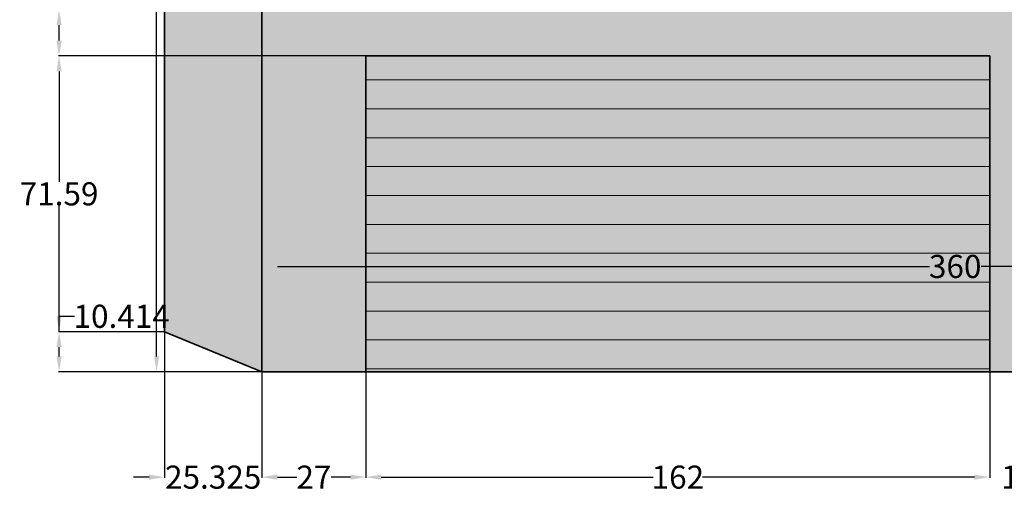
# Model space of a CAD drawing. Units: inches. Extents: x 184 to 649, y 215 to 818.
# Tile 1 of 9: x 186 to 442, y 215 to 338. Entities that reach past the tile are written whole.
import ezdxf

# ---------------------------------------------------------------- set-up
doc = ezdxf.new("R2010")
doc.units = ezdxf.units.IN
doc.header["$MEASUREMENT"] = 0
for name, color, linetype, lineweight in [('A-ANNO-DIMS', 2, 'Continuous', 18), ('A-ELEV', 7, 'Continuous', 35), ('A-ELEV-FILL', 9, 'Continuous', 13), ('A-ELEV-PATT', 8, 'Continuous', 13)]:
    doc.layers.add(name, color=color, linetype=linetype, lineweight=lineweight)
doc.styles.get("Standard").update_dxf_attribs({"font": 'arial.ttf'})
doc.dimstyles.get("Standard").update_dxf_attribs({"dimtxt": 6, "dimasz": 4, "dimexe": 0.18, "dimexo": 0.0625, "dimgap": 0.09, "dimtad": 0, "dimtih": 1, "dimtoh": 1, "dimdec": 0, "dimzin": 0, "dimdsep": 46, "dimlunit": 3, "dimtxsty": 'Standard', "dimcen": 0.09, "dimadec": 0, "dimazin": 0, "dimtfac": 1, "dimtdec": 0, "dimtofl": 0, "dimtmove": 0, "dimatfit": 3, "dimfxl": 1, "dimtolj": 1, "dimtzin": 0, "dimarcsym": 0})

# ---------------------------------------------------------------- blocks, each defined once
blk = doc.blocks.new('*D9')
at = {"layer": 'A-ANNO-DIMS', "color": 0, "lineweight": -2, "transparency": 16777216}
for p, q in [((248.97, 246.79), (248.97, 274.26)), ((252.97, 274.08), (422.27, 274.08)), ((604.97, 274.08), (435.68, 274.08)), ((608.97, 246.79), (608.97, 274.26))]:
    blk.add_line(p, q, dxfattribs=at)
at = {"layer": 'A-ANNO-DIMS', "color": 0, "transparency": 16777216}
for points in [[(252.97, 274.74), (252.97, 273.41), (248.97, 274.08)], [(604.97, 274.74), (604.97, 273.41), (608.97, 274.08)]]:
    blk.add_solid(points, dxfattribs=at)
at = {"layer": 'Defpoints', "color": 0, "transparency": 16777216}
for p in [(608.97, 274.08), (248.97, 246.73), (608.97, 246.73)]:
    blk.add_point(p, dxfattribs=at)
at = {"layer": 'A-ANNO-DIMS', "color": 0, "transparency": 16777216, "insert": (428.97, 274.08), "char_height": 6, "attachment_point": 5}
blk.add_mtext('\\A1;360', dxfattribs=at)
blk = doc.blocks.new('*D10')
at = {"layer": 'A-ANNO-DIMS', "color": 0, "lineweight": -2, "transparency": 16777216}
for p, q in [((248.91, 786.73), (221.44, 786.73)), ((221.62, 782.73), (221.62, 519.88)), ((221.62, 250.73), (221.62, 513.57)), ((248.91, 246.73), (221.44, 246.73))]:
    blk.add_line(p, q, dxfattribs=at)
at = {"layer": 'A-ANNO-DIMS', "color": 0, "transparency": 16777216}
for points in [[(220.96, 782.73), (222.29, 782.73), (221.62, 786.73)], [(220.96, 250.73), (222.29, 250.73), (221.62, 246.73)]]:
    blk.add_solid(points, dxfattribs=at)
at = {"layer": 'Defpoints', "color": 0, "transparency": 16777216}
for p in [(221.62, 786.73), (248.97, 786.73), (248.97, 246.73)]:
    blk.add_point(p, dxfattribs=at)
at = {"layer": 'A-ANNO-DIMS', "color": 0, "transparency": 16777216, "insert": (221.62, 516.73), "char_height": 6, "attachment_point": 5}
blk.add_mtext('\\A1;540', dxfattribs=at)
blk = doc.blocks.new('*D11')
at = {"layer": 'A-ANNO-DIMS', "color": 0, "lineweight": -2, "transparency": 16777216}
for p, q in [((223.65, 257.08), (223.65, 219.2)), ((248.97, 246.66), (248.97, 219.2)), ((219.65, 219.38), (215.65, 219.38)), ((252.97, 219.38), (256.97, 219.38))]:
    blk.add_line(p, q, dxfattribs=at)
at = {"layer": 'A-ANNO-DIMS', "color": 0, "transparency": 16777216}
for points in [[(219.65, 220.04), (219.65, 218.71), (223.65, 219.38)], [(252.97, 220.04), (252.97, 218.71), (248.97, 219.38)]]:
    blk.add_solid(points, dxfattribs=at)
at = {"layer": 'Defpoints', "color": 0, "transparency": 16777216}
for p in [(223.65, 257.14), (248.97, 246.73), (248.97, 219.38)]:
    blk.add_point(p, dxfattribs=at)
at = {"layer": 'A-ANNO-DIMS', "color": 0, "transparency": 16777216, "insert": (236.31, 219.38), "char_height": 6, "attachment_point": 5}
blk.add_mtext('\\A1;25.325', dxfattribs=at)
blk = doc.blocks.new('*D12')
at = {"layer": 'A-ANNO-DIMS', "color": 0, "lineweight": -2, "transparency": 16777216}
for p, q in [((248.97, 246.66), (248.97, 219.2)), ((275.97, 246.66), (275.97, 219.2)), ((252.97, 219.38), (258.03, 219.38)), ((271.97, 219.38), (266.91, 219.38))]:
    blk.add_line(p, q, dxfattribs=at)
at = {"layer": 'A-ANNO-DIMS', "color": 0, "transparency": 16777216}
for points in [[(252.97, 220.04), (252.97, 218.71), (248.97, 219.38)], [(271.97, 220.04), (271.97, 218.71), (275.97, 219.38)]]:
    blk.add_solid(points, dxfattribs=at)
at = {"layer": 'Defpoints', "color": 0, "transparency": 16777216}
for p in [(248.97, 246.73), (275.97, 246.73), (275.97, 219.38)]:
    blk.add_point(p, dxfattribs=at)
at = {"layer": 'A-ANNO-DIMS', "color": 0, "transparency": 16777216, "insert": (262.47, 219.38), "char_height": 6, "attachment_point": 5}
blk.add_mtext('\\A1;27', dxfattribs=at)
blk = doc.blocks.new('*D13')
at = {"layer": 'A-ANNO-DIMS', "color": 0, "lineweight": -2, "transparency": 16777216}
for p, q in [((275.97, 246.66), (275.97, 219.2)), ((437.97, 246.66), (437.97, 219.2)), ((279.97, 219.38), (350.57, 219.38)), ((433.97, 219.38), (363.38, 219.38))]:
    blk.add_line(p, q, dxfattribs=at)
at = {"layer": 'A-ANNO-DIMS', "color": 0, "transparency": 16777216}
for points in [[(279.97, 220.04), (279.97, 218.71), (275.97, 219.38)], [(433.97, 220.04), (433.97, 218.71), (437.97, 219.38)]]:
    blk.add_solid(points, dxfattribs=at)
at = {"layer": 'Defpoints', "color": 0, "transparency": 16777216}
for p in [(275.97, 246.73), (437.97, 246.73), (437.97, 219.38)]:
    blk.add_point(p, dxfattribs=at)
at = {"layer": 'A-ANNO-DIMS', "color": 0, "transparency": 16777216, "insert": (356.97, 219.38), "char_height": 6, "attachment_point": 5}
blk.add_mtext('\\A1;162', dxfattribs=at)
blk = doc.blocks.new('*D14')
at = {"layer": 'A-ANNO-DIMS', "color": 0, "lineweight": -2, "transparency": 16777216}
for p, q in [((452.97, 282.66), (452.97, 219.2)), ((437.97, 246.66), (437.97, 219.2)), ((433.97, 219.38), (429.97, 219.38)), ((456.97, 219.38), (460.97, 219.38))]:
    blk.add_line(p, q, dxfattribs=at)
at = {"layer": 'A-ANNO-DIMS', "color": 0, "transparency": 16777216}
for points in [[(433.97, 220.04), (433.97, 218.71), (437.97, 219.38)], [(456.97, 220.04), (456.97, 218.71), (452.97, 219.38)]]:
    blk.add_solid(points, dxfattribs=at)
at = {"layer": 'Defpoints', "color": 0, "transparency": 16777216}
for p in [(452.97, 282.73), (437.97, 246.73), (452.97, 219.38)]:
    blk.add_point(p, dxfattribs=at)
at = {"layer": 'A-ANNO-DIMS', "color": 0, "transparency": 16777216, "insert": (445.47, 219.38), "char_height": 6, "attachment_point": 5}
blk.add_mtext('\\A1;15', dxfattribs=at)
blk = doc.blocks.new('*D30')
at = {"layer": 'A-ANNO-DIMS', "color": 0, "lineweight": -2, "transparency": 16777216}
for p, q in [((196.3, 257.14), (196.3, 261.14)), ((196.3, 261.14), (200.3, 261.14)), ((223.58, 257.14), (196.12, 257.14)), ((196.3, 250.73), (196.3, 253.14)), ((248.91, 246.73), (196.12, 246.73))]:
    blk.add_line(p, q, dxfattribs=at)
at = {"layer": 'A-ANNO-DIMS', "color": 0, "transparency": 16777216}
for points in [[(195.63, 253.14), (196.96, 253.14), (196.3, 257.14)], [(195.63, 250.73), (196.96, 250.73), (196.3, 246.73)]]:
    blk.add_solid(points, dxfattribs=at)
at = {"layer": 'Defpoints', "color": 0, "transparency": 16777216}
for p in [(196.3, 257.14), (223.65, 257.14), (248.97, 246.73)]:
    blk.add_point(p, dxfattribs=at)
at = {"layer": 'A-ANNO-DIMS', "color": 0, "transparency": 16777216, "insert": (212.55, 261.14), "char_height": 6, "attachment_point": 5}
blk.add_mtext('\\A1;10.414', dxfattribs=at)
blk = doc.blocks.new('*D31')
at = {"layer": 'A-ANNO-DIMS', "color": 0, "lineweight": -2, "transparency": 16777216}
for p, q in [((275.91, 328.73), (196.12, 328.73)), ((196.3, 324.73), (196.3, 296.09)), ((196.3, 261.14), (196.3, 289.78)), ((223.58, 257.14), (196.12, 257.14))]:
    blk.add_line(p, q, dxfattribs=at)
at = {"layer": 'A-ANNO-DIMS', "color": 0, "transparency": 16777216}
for points in [[(195.63, 324.73), (196.96, 324.73), (196.3, 328.73)], [(195.63, 261.14), (196.96, 261.14), (196.3, 257.14)]]:
    blk.add_solid(points, dxfattribs=at)
at = {"layer": 'Defpoints', "color": 0, "transparency": 16777216}
for p in [(196.3, 328.73), (275.97, 328.73), (223.65, 257.14)]:
    blk.add_point(p, dxfattribs=at)
at = {"layer": 'A-ANNO-DIMS', "color": 0, "transparency": 16777216, "insert": (196.3, 292.93), "char_height": 6, "attachment_point": 5}
blk.add_mtext('\\A1;71.59', dxfattribs=at)
blk = doc.blocks.new('*D32')
at = {"layer": 'A-ANNO-DIMS', "color": 0, "lineweight": -2, "transparency": 16777216}
for p, q in [((196.3, 340.73), (196.3, 344.73)), ((196.3, 344.73), (200.3, 344.73)), ((275.91, 340.73), (196.12, 340.73)), ((196.3, 332.73), (196.3, 336.73)), ((275.91, 328.73), (196.12, 328.73))]:
    blk.add_line(p, q, dxfattribs=at)
at = {"layer": 'A-ANNO-DIMS', "color": 0, "transparency": 16777216}
for points in [[(195.63, 336.73), (196.96, 336.73), (196.3, 340.73)], [(195.63, 332.73), (196.96, 332.73), (196.3, 328.73)]]:
    blk.add_solid(points, dxfattribs=at)
at = {"layer": 'Defpoints', "color": 0, "transparency": 16777216}
for p in [(196.3, 340.73), (275.97, 340.73), (275.97, 328.73)]:
    blk.add_point(p, dxfattribs=at)
at = {"layer": 'A-ANNO-DIMS', "color": 0, "transparency": 16777216, "insert": (204.37, 344.73), "char_height": 6, "attachment_point": 5}
blk.add_mtext('\\A1;12', dxfattribs=at)

msp = doc.modelspace()

# ---------------------------------------------------------------- hatches: boundary and pattern name
at = {"layer": 'A-ELEV-FILL'}
h = msp.add_hatch(color=256, dxfattribs=at)
h.dxf.hatch_style = 1
h.paths.add_polyline_path([(248.9726, 786.7265), (223.6471, 761.141), (223.6471, 257.141), (248.9726, 246.7265)])
h = msp.add_hatch(color=256, dxfattribs=at)
h.dxf.hatch_style = 1
h.paths.add_polyline_path([(452.9726, 369.7265), (248.9726, 369.7265), (248.9726, 246.7265), (275.9726, 246.7265), (275.9726, 328.7265), (437.9726, 328.7265), (437.9726, 246.7265), (446.6666, 246.7265), (452.9726, 282.7265)])
h.paths.add_polyline_path([(275.9726, 340.7265), (275.9726, 354.7265), (437.9726, 354.7265), (437.9726, 340.7265)], flags=16)
h.paths.add_polyline_path([(452.9726, 510.7265), (260.9726, 510.7265), (260.9726, 642.7265), (260.9726, 699.7265), (367.0226, 699.7265), (373.9381, 706.7265), (260.9726, 706.7265), (260.9726, 715.7265), (382.8295, 715.7265), (389.745, 722.7265), (260.9726, 722.7265), (260.9726, 731.7265), (398.6364, 731.7265), (405.5519, 738.7265), (260.9726, 738.7265), (260.9726, 747.7265), (414.4433, 747.7265), (421.3588, 754.7265), (260.9726, 754.7265), (260.9726, 763.7265), (430.2502, 763.7265), (437.1657, 770.7265), (260.9726, 770.7265), (260.9726, 779.7265), (446.057, 779.7265), (452.9726, 786.7265), (248.9726, 786.7265), (248.9726, 369.7265), (260.9726, 369.7265), (260.9726, 498.7265), (452.9726, 498.7265)])
h = msp.add_hatch(color=256, dxfattribs=at)
h.dxf.hatch_style = 1
h.paths.add_polyline_path([(380.9726, 453.5037), (422.2268, 453.5037), (422.2268, 474.7265), (260.9726, 474.7265), (260.9726, 369.7265), (291.9998, 369.7265), (291.9998, 453.5037), (339.9998, 453.5037), (339.9998, 369.7265), (380.9726, 369.7265)])
h.paths.add_polyline_path([(437.9726, 328.7265), (275.9726, 328.7265), (275.9726, 246.7265), (437.9726, 246.7265)])
h.paths.add_polyline_path([(581.9726, 759.7265), (521.9726, 759.7265), (521.9726, 441.2233), (581.9726, 441.2233)])
h.paths.add_polyline_path([(560.9726, 582.4749), (560.9726, 477.2233), (542.9726, 477.2233), (542.9726, 582.4749)], flags=16)
h.paths.add_polyline_path([(560.9726, 618.4749), (542.9726, 618.4749), (542.9726, 723.7265), (560.9726, 723.7265)], flags=16)
at = {"layer": 'A-ELEV-PATT'}
h = msp.add_hatch(dxfattribs=at)
h.set_pattern_fill('ANSI31', color=256, scale=60, angle=135)
h.paths.add_polyline_path([(437.9726, 328.7265), (275.9726, 328.7265), (275.9726, 246.7265), (437.9726, 246.7265)])

# ---------------------------------------------------------------- linework, layer by layer
at = {"layer": 'A-ELEV'}
for p, q in [((248.9726, 786.7265), (248.9726, 246.7265)), ((223.6471, 761.141), (223.6471, 257.141)), ((437.9726, 328.7265), (275.9726, 328.7265)), ((275.9726, 328.7265), (275.9726, 246.7265)), ((437.9726, 246.7265), (437.9726, 328.7265)), ((223.6471, 257.141), (248.9726, 246.7265)), ((248.9726, 246.7265), (608.9726, 246.7265))]:
    msp.add_line(p, q, dxfattribs=at)

# ---------------------------------------------------------------- dimensions: what is measured, and where the dimension line sits
at = {"layer": 'A-ANNO-DIMS'}
for base, p1, p2, override, picture, middle in [((221.6226, 786.7265), (248.9726, 246.7265), (248.9726, 786.7265), {"dimdec": 0, "dimlfac": 1, "dimrnd": 0, "dimzin": 0, "dimdsep": 46, "dimlunit": 2}, '*D10', (221.6226, 516.7265)), ((196.2971, 340.7265), (275.9726, 328.7265), (275.9726, 340.7265), {"dimdec": 0, "dimlfac": 1, "dimrnd": 0, "dimzin": 0, "dimdsep": 46, "dimlunit": 2}, '*D32', (204.3714, 344.7265)), ((196.2971, 328.7265), (223.6471, 257.141), (275.9726, 328.7265), {"dimdec": 2, "dimlfac": 1, "dimrnd": 0, "dimzin": 0, "dimdsep": 46, "dimlunit": 2}, '*D31', (196.2971, 292.9338)), ((196.29709, 257.14099), (248.97256, 246.72655), (223.64709, 257.14099), {"dimdec": 3, "dimlfac": 1, "dimrnd": 0, "dimzin": 0, "dimdsep": 46, "dimlunit": 2}, '*D30', (212.54671, 261.14099))]:
    dim = msp.add_linear_dim(base=base, p1=p1, p2=p2, angle=90, dimstyle='Standard', override=override, dxfattribs=at)
    dim.commit()
    dim.dimension.update_dxf_attribs({"geometry": picture, "text_midpoint": middle})
for base, p1, p2, override, picture, middle in [((452.9726, 219.3765), (437.9726, 246.7265), (452.9726, 282.7265), {"dimdec": 0, "dimlfac": 1, "dimrnd": 0, "dimzin": 0, "dimdsep": 46, "dimlunit": 2}, '*D14', (445.4726, 219.3765)), ((608.9726, 274.0765), (248.9726, 246.7265), (608.9726, 246.7265), {"dimdec": 0, "dimlfac": 1, "dimrnd": 0, "dimzin": 0, "dimdsep": 46, "dimlunit": 2}, '*D9', (428.9726, 274.0765)), ((248.97256, 219.37655), (223.64709, 257.14099), (248.97256, 246.72655), {"dimdec": 3, "dimlfac": 1, "dimrnd": 0, "dimzin": 0, "dimdsep": 46, "dimlunit": 2}, '*D11', (236.30982, 219.37655)), ((275.9726, 219.3765), (248.9726, 246.7265), (275.9726, 246.7265), {"dimdec": 0, "dimlfac": 1, "dimrnd": 0, "dimzin": 0, "dimdsep": 46, "dimlunit": 2}, '*D12', (262.4726, 219.3765)), ((437.9726, 219.3765), (275.9726, 246.7265), (437.9726, 246.7265), {"dimdec": 0, "dimlfac": 1, "dimrnd": 0, "dimzin": 0, "dimdsep": 46, "dimlunit": 2}, '*D13', (356.9726, 219.3765))]:
    dim = msp.add_linear_dim(base=base, p1=p1, p2=p2, dimstyle='Standard', override=override, dxfattribs=at)
    dim.commit()
    dim.dimension.update_dxf_attribs({"geometry": picture, "text_midpoint": middle})

doc.saveas('drawing.dxf')
